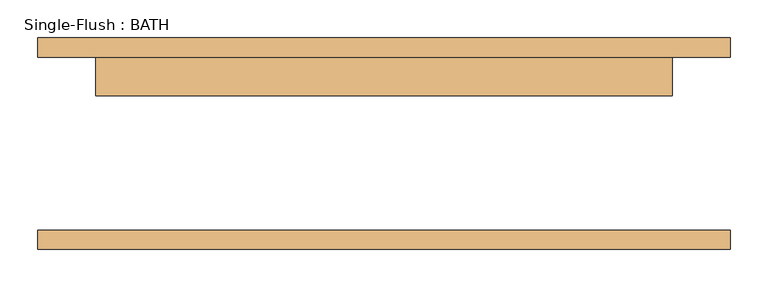
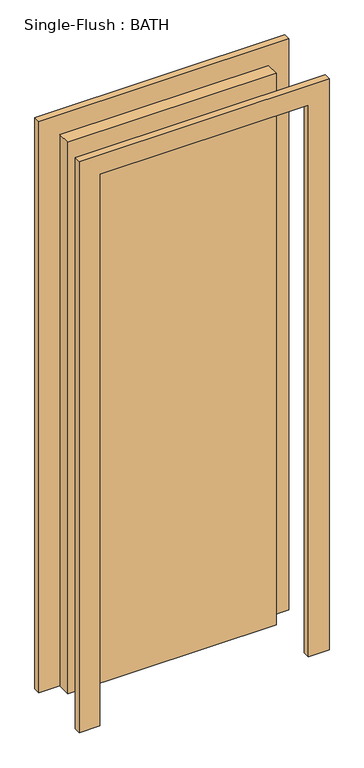
"""IFC4 building model written with IfcOpenShell, lengths in millimetres: door geometry, Single-Flush : BATH."""

from ifc_helpers import new_model, si_unit, frame, origin, origin_with_axes, place, context, project, spatial, polyline, outline, extrude, source, transform, mapped, element, save


def single_flush_bath_bb98abfd(model_context):
    return source(origin(), model_context, "Body", "SweptSolid", [
        extrude(outline(polyline([(2209.8, -457.2), (0.0, -457.2), (0.0, -381.0), (2133.6, -381.0), (2133.6, 381.0), (0.0, 381.0), (0.0, 457.2), (2209.8, 457.2), (2209.8, -457.2)])), frame((0.0, 114.3, 0.0), z_axis=(0.0, 1.0, 0.0), x_axis=(0.0, 0.0, 1.0)), (0.0, 0.0, 1.0), 25.4),
        extrude(outline(polyline([(2209.8, 457.2), (2209.8, -457.2), (0.0, -457.2), (0.0, -381.0), (2133.6, -381.0), (2133.6, 381.0), (0.0, 381.0), (0.0, 457.2), (2209.8, 457.2)])), frame((0.0, -139.7, 0.0), z_axis=(0.0, 1.0, 0.0), x_axis=(0.0, 0.0, 1.0)), (0.0, 0.0, 1.0), 25.4),
        extrude(outline(polyline([(381.0, 63.5), (-381.0, 63.5), (-381.0, 114.3), (381.0, 114.3), (381.0, 63.5)])), origin_with_axes(), (0.0, 0.0, 1.0), 2133.6),
    ])


if __name__ == "__main__":
    model = new_model("IFC4")
    model_context = context("Model", 3, world=origin())
    ifc_project = project(units=[si_unit("LENGTHUNIT", "METRE", prefix="MILLI")], contexts=[model_context])
    site = spatial("IfcSite", under=ifc_project)
    building = spatial("IfcBuilding", under=site)
    placement = place(None, origin())
    single_flush_bath_shape = single_flush_bath_bb98abfd(model_context)
    element("IfcDoor", 1, ObjectType="Single-Flush : BATH", at=placement, inside=building, context=model_context, shape_type="MappedRepresentation", body=[
        mapped(single_flush_bath_shape, transform((0.0, 0.0, 0.0), x_axis=(1.0, 0.0, 0.0), y_axis=(0.0, 1.0, 0.0), z_axis=(0.0, 0.0, 1.0))),
    ])
    save(model, "model.ifc")

# Revit data of these elements
# Type "Single-Flush : BATH"
#   Type Mark = "9"
#   Construction Type Id = "MDOOR"
#   Assembly Code = "C1020"
#   Analytic Construction = "Metal"
#   Thickness = 0' - 2"
#   Heat Transfer Coefficient (U) = 0.651978 BTU/(h·ft²·°F)
#   Height = 7' - 0"
#   Trim Projection Ext = 0' - 1"
#   Trim Projection Int = 0' - 1"
#   Trim Width = 0' - 3"
#   Width = 2' - 6"
#   Define Thermal Properties by = 1
#   Door Material = Door - Panel
#   Frame Material = Door - Frame
#   Visual Light Transmittance = 0
#   Solar Heat Gain Coefficient = 0
#   Function = (empty or 0)
#   Wall Closure = (empty or 0)
# Element 1 (IfcDoor, "Single-Flush : BATH")
#   Materials on its faces: "Door - Frame", "Door - Panel"
# Materials
#   "Door - Panel": class "Wood", colour RGB 210 159 95, transparency 0, Cost = 0
#   "Door - Frame": colour RGB 118 70 51, transparency 0, Cost = 0
